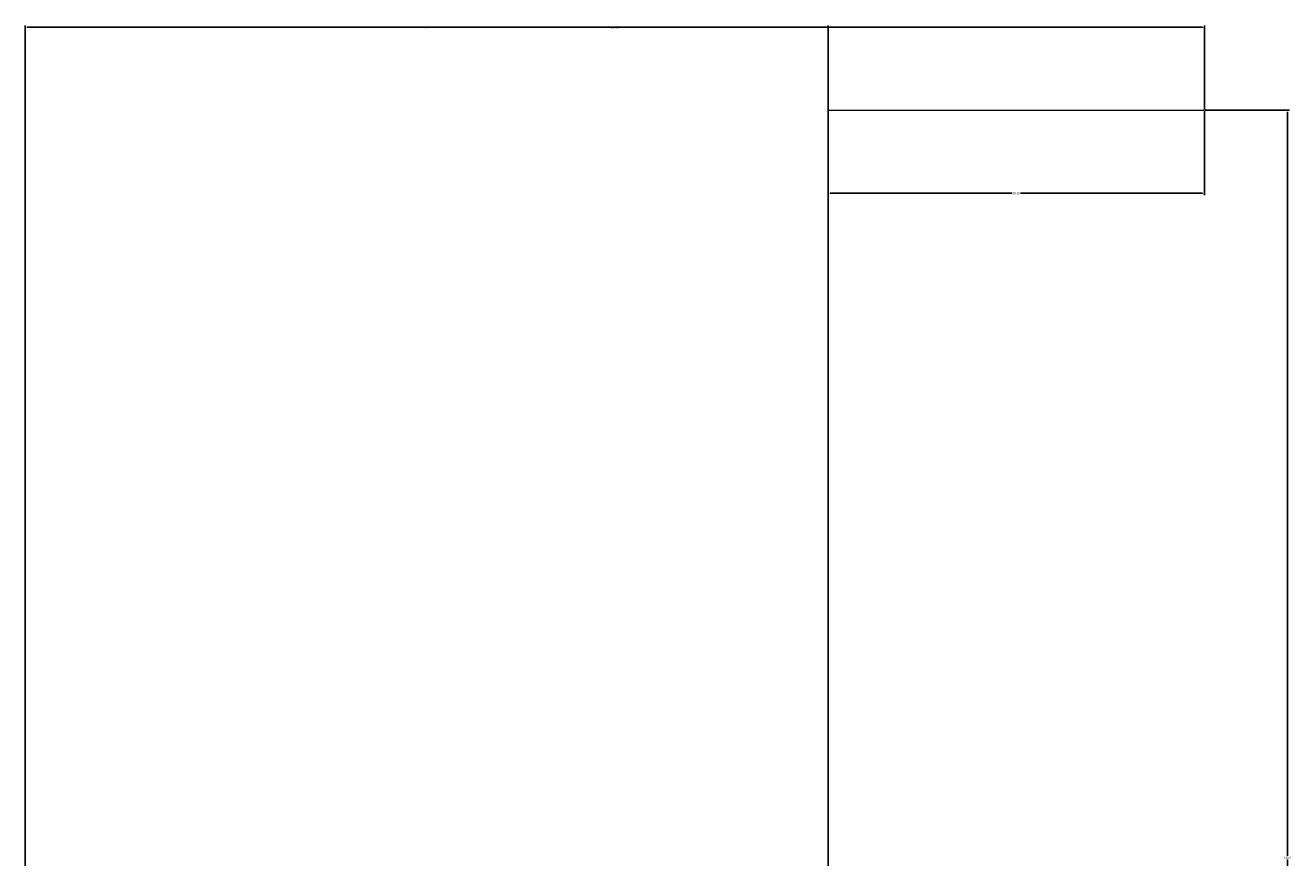
# Model space of a CAD drawing. Units: millimetres. Extents: x 118 to 244, y 285 to 440.
# Tile 4 of 4: x 126 to 244, y 362 to 440. Entities that reach past the tile are written whole.
import ezdxf

# ---------------------------------------------------------------- set-up
doc = ezdxf.new("R2010")
doc.units = ezdxf.units.MM
doc.layers.add('M-CONS', color=8, linetype='Continuous', lineweight=13)
doc.layers.add('M-DIMS', color=2, linetype='Continuous', lineweight=18)
doc.styles.get("Standard").update_dxf_attribs({"font": 'arial.ttf'})
doc.dimstyles.get("Standard").update_dxf_attribs({"dimtxt": 0.18, "dimasz": 0.18, "dimexe": 0.18, "dimexo": 0.0625, "dimgap": 0.09, "dimtad": 0, "dimtih": 1, "dimtoh": 1, "dimdec": 4, "dimzin": 0, "dimdsep": 46, "dimtxsty": 'Standard', "dimcen": 0.09, "dimadec": 0, "dimazin": 0, "dimtfac": 1, "dimtdec": 4, "dimtofl": 0, "dimtmove": 0, "dimatfit": 3, "dimfxl": 1, "dimtolj": 1, "dimtzin": 0, "dimarcsym": 0})

# ---------------------------------------------------------------- blocks, each defined once
blk = doc.blocks.new('*D3')
at = {"layer": 'Defpoints', "color": 0, "transparency": 16777216}
for p in [(200.52, 439.79), (125.52, 346.44), (200.52, 346.44)]:
    blk.add_point(p, dxfattribs=at)
at = {"layer": 'M-DIMS', "color": 0, "lineweight": -2, "transparency": 16777216}
for p, q in [((125.52, 346.5), (125.52, 439.97)), ((125.7, 439.79), (162.81, 439.79)), ((200.34, 439.79), (163.24, 439.79)), ((200.52, 346.5), (200.52, 439.97))]:
    blk.add_line(p, q, dxfattribs=at)
at = {"layer": 'M-DIMS', "color": 0, "transparency": 16777216}
for points in [[(125.7, 439.82), (125.7, 439.76), (125.52, 439.79)], [(200.34, 439.82), (200.34, 439.76), (200.52, 439.79)]]:
    blk.add_solid(points, dxfattribs=at)
at = {"layer": 'M-DIMS', "color": 0, "transparency": 16777216, "insert": (163.02, 439.79), "char_height": 0.18, "attachment_point": 5}
blk.add_mtext('\\A1;75', dxfattribs=at)
blk = doc.blocks.new('*D8')
at = {"layer": 'Defpoints', "color": 0, "transparency": 16777216}
for p in [(200.52, 432.04), (235.68, 432.04), (200.52, 424.29)]:
    blk.add_point(p, dxfattribs=at)
at = {"layer": 'M-DIMS', "color": 0, "lineweight": -2, "transparency": 16777216}
for p, q in [((200.52, 431.98), (200.52, 424.11)), ((235.68, 431.98), (235.68, 424.11)), ((200.7, 424.29), (217.71, 424.29)), ((235.5, 424.29), (218.49, 424.29))]:
    blk.add_line(p, q, dxfattribs=at)
at = {"layer": 'M-DIMS', "color": 0, "transparency": 16777216}
for points in [[(200.7, 424.32), (200.7, 424.26), (200.52, 424.29)], [(235.5, 424.32), (235.5, 424.26), (235.68, 424.29)]]:
    blk.add_solid(points, dxfattribs=at)
at = {"layer": 'M-DIMS', "color": 0, "transparency": 16777216, "insert": (218.1, 424.29), "char_height": 0.18, "attachment_point": 5}
blk.add_mtext('\\A1;35.15', dxfattribs=at)
blk = doc.blocks.new('*D9')
at = {"layer": 'Defpoints', "color": 0, "transparency": 16777216}
for p in [(235.68, 439.79), (235.68, 432.04), (125.52, 346.44)]:
    blk.add_point(p, dxfattribs=at)
at = {"layer": 'M-DIMS', "color": 0, "lineweight": -2, "transparency": 16777216}
for p, q in [((125.52, 346.5), (125.52, 439.97)), ((125.7, 439.79), (180.14, 439.79)), ((235.5, 439.79), (181.06, 439.79)), ((235.68, 432.11), (235.68, 439.97))]:
    blk.add_line(p, q, dxfattribs=at)
at = {"layer": 'M-DIMS', "color": 0, "transparency": 16777216}
for points in [[(125.7, 439.82), (125.7, 439.76), (125.52, 439.79)], [(235.5, 439.82), (235.5, 439.76), (235.68, 439.79)]]:
    blk.add_solid(points, dxfattribs=at)
at = {"layer": 'M-DIMS', "color": 0, "transparency": 16777216, "insert": (180.6, 439.79), "char_height": 0.18, "attachment_point": 5}
blk.add_mtext('\\A1;110.15', dxfattribs=at)
blk = doc.blocks.new('*D10')
at = {"layer": 'Defpoints', "color": 0, "transparency": 16777216}
for p in [(235.68, 432.04), (243.43, 432.04), (125.52, 292.44)]:
    blk.add_point(p, dxfattribs=at)
at = {"layer": 'M-DIMS', "color": 0, "lineweight": -2, "transparency": 16777216}
for p, q in [((235.74, 432.04), (243.61, 432.04)), ((243.43, 431.86), (243.43, 362.42)), ((243.43, 292.62), (243.43, 362.06)), ((125.59, 292.44), (243.61, 292.44))]:
    blk.add_line(p, q, dxfattribs=at)
at = {"layer": 'M-DIMS', "color": 0, "transparency": 16777216}
for points in [[(243.4, 431.86), (243.46, 431.86), (243.43, 432.04)], [(243.4, 292.62), (243.46, 292.62), (243.43, 292.44)]]:
    blk.add_solid(points, dxfattribs=at)
at = {"layer": 'M-DIMS', "color": 0, "transparency": 16777216, "insert": (243.43, 362.24), "char_height": 0.18, "attachment_point": 5}
blk.add_mtext('\\A1;139.6', dxfattribs=at)

msp = doc.modelspace()

# ---------------------------------------------------------------- linework, layer by layer
at = {"layer": 'M-CONS'}
msp.add_line((200.5241, 432.0445), (235.6768, 432.0445), dxfattribs=at)

# ---------------------------------------------------------------- dimensions: what is measured, and where the dimension line sits
at = {"layer": 'M-DIMS'}
for base, p2, override, picture, middle in [((200.5241, 439.7945), (200.5241, 346.4369), {"dimdec": 0, "dimlfac": 1, "dimrnd": 0, "dimzin": 0, "dimdsep": 46, "dimlunit": 2}, '*D3', (163.0241, 439.7945)), ((235.6768, 439.7945), (235.6768, 432.0445), {"dimdec": 2, "dimlfac": 1, "dimrnd": 0, "dimzin": 0, "dimdsep": 46, "dimlunit": 2}, '*D9', (180.6005, 439.7945))]:
    dim = msp.add_linear_dim(base=base, p1=(125.5241, 346.4369), p2=p2, dimstyle='Standard', override=override, dxfattribs=at)
    dim.commit()
    dim.dimension.update_dxf_attribs({"geometry": picture, "text_midpoint": middle})
for base, p1, p2, angle, override, picture, middle in [((243.4268, 432.0445), (125.5241, 292.4369), (235.6768, 432.0445), 90, {"dimdec": 1, "dimlfac": 1, "dimrnd": 0, "dimzin": 0, "dimdsep": 46, "dimlunit": 2}, '*D10', (243.4268, 362.2407)), ((200.5241, 424.2945), (235.6768, 432.0445), (200.5241, 432.0445), 180, {"dimdec": 2, "dimlfac": 1, "dimrnd": 0, "dimzin": 0, "dimdsep": 46, "dimlunit": 2}, '*D8', (218.1005, 424.2945))]:
    dim = msp.add_linear_dim(base=base, p1=p1, p2=p2, angle=angle, dimstyle='Standard', override=override, dxfattribs=at)
    dim.commit()
    dim.dimension.update_dxf_attribs({"geometry": picture, "text_midpoint": middle})

doc.saveas('drawing.dxf')
